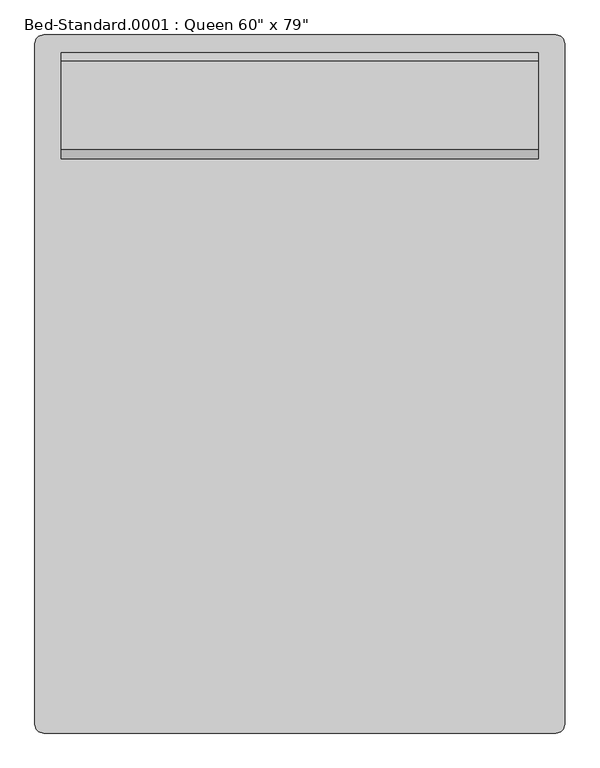
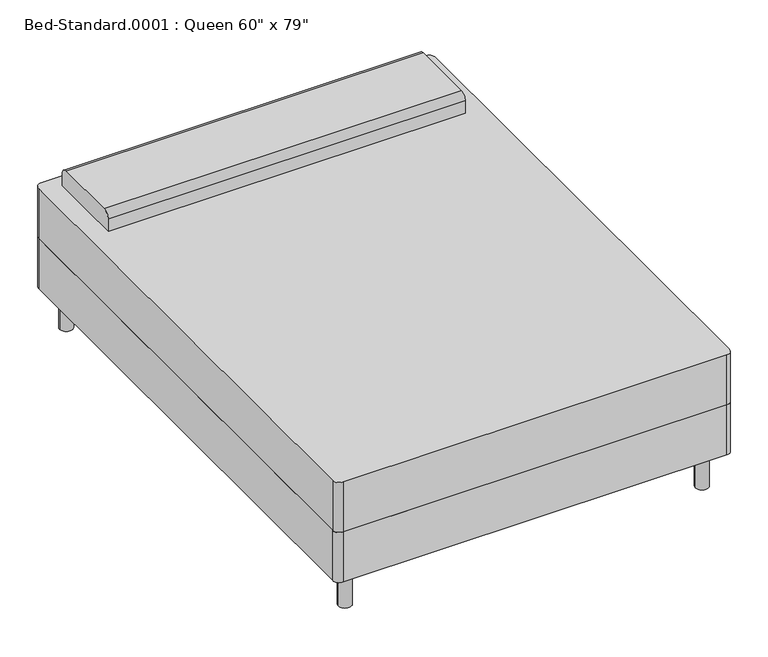
"""IFC4 building model written with IfcOpenShell, lengths in millimetres: furniture geometry."""

from ifc_helpers import new_model, si_unit, point, frame, frame_2d, origin, origin_with_axes, place, context, project, spatial, polyline, circle_curve, trimmed, segment, composite_curve, outline, extrude, source, transform, mapped, element, save


def furniture_e1791683(model_context):
    return source(origin(), model_context, "Body", "SweptSolid", [
        extrude(outline(composite_curve([segment(polyline([(-490.5114754, -1023.495082), (-490.5114754, 932.304918)]), True, "CONTINUOUS"), segment(trimmed(circle_curve(frame_2d((-465.1114754, 932.304918)), 25.4), [point((-490.5114754, 932.304918))], [point((-465.1114754, 957.704918))], False, "CARTESIAN"), True, "CONTINUOUS"), segment(polyline([(-465.1114754, 957.704918), (1008.0885246, 957.704918)]), True, "CONTINUOUS"), segment(trimmed(circle_curve(frame_2d((1008.0885246, 932.304918)), 25.4), [point((1008.0885246, 957.704918))], [point((1033.4885246, 932.304918))], False, "CARTESIAN"), True, "CONTINUOUS"), segment(polyline([(1033.4885246, 932.304918), (1033.4885246, -1023.495082)]), True, "CONTINUOUS"), segment(trimmed(circle_curve(frame_2d((1008.0885246, -1023.495082)), 25.4), [point((1033.4885246, -1023.495082))], [point((1008.0885246, -1048.895082))], False, "CARTESIAN"), True, "CONTINUOUS"), segment(polyline([(1008.0885246, -1048.895082), (-465.1114754, -1048.895082)]), True, "CONTINUOUS"), segment(trimmed(circle_curve(frame_2d((-465.1114754, -1023.495082)), 25.4), [point((-465.1114754, -1048.895082))], [point((-490.5114754, -1023.495082))], False, "CARTESIAN"), True, "CONTINUOUS")], self_intersect=False)), frame((0.0, 0.0, 152.4), z_axis=(0.0, 0.0, 1.0), x_axis=(1.0, 0.0, 0.0)), (0.0, 0.0, 1.0), 203.2),
        extrude(outline(composite_curve([segment(polyline([(602.104918, 558.8), (602.104918, 609.6)]), True, "CONTINUOUS"), segment(trimmed(circle_curve(frame_2d((627.504918, 609.6)), 25.4), [point((602.104918, 609.6))], [point((627.504918, 635.0))], False, "CARTESIAN"), True, "CONTINUOUS"), segment(polyline([(627.504918, 635.0), (881.504918, 635.0)]), True, "CONTINUOUS"), segment(trimmed(circle_curve(frame_2d((881.504918, 609.6)), 25.4), [point((881.504918, 635.0))], [point((906.904918, 609.6))], False, "CARTESIAN"), True, "CONTINUOUS"), segment(polyline([(906.904918, 609.6), (906.904918, 558.8), (602.104918, 558.8)]), True, "CONTINUOUS")], self_intersect=False)), frame((-414.3114754, 0.0, 0.0), z_axis=(1.0, 0.0, 0.0), x_axis=(0.0, 1.0, 0.0)), (0.0, 0.0, 1.0), 1371.6),
        extrude(outline(composite_curve([segment(trimmed(circle_curve(frame_2d((-414.3114754, 881.504918)), 25.4), [point((-439.7114754, 881.504918))], [point((-388.9114754, 881.504918))], False, "CARTESIAN"), True, "CONTINUOUS"), segment(trimmed(circle_curve(frame_2d((-414.3114754, 881.504918)), 25.4), [point((-388.9114754, 881.504918))], [point((-439.7114754, 881.504918))], False, "CARTESIAN"), True, "CONTINUOUS")], self_intersect=False)), origin_with_axes(), (0.0, 0.0, 1.0), 152.4),
        extrude(outline(composite_curve([segment(trimmed(circle_curve(frame_2d((957.2885246, 881.504918)), 25.4), [point((931.8885246, 881.504918))], [point((982.6885246, 881.504918))], False, "CARTESIAN"), True, "CONTINUOUS"), segment(trimmed(circle_curve(frame_2d((957.2885246, 881.504918)), 25.4), [point((982.6885246, 881.504918))], [point((931.8885246, 881.504918))], False, "CARTESIAN"), True, "CONTINUOUS")], self_intersect=False)), origin_with_axes(), (0.0, 0.0, 1.0), 152.4),
        extrude(outline(composite_curve([segment(trimmed(circle_curve(frame_2d((957.2885246, -972.695082)), 25.4), [point((931.8885246, -972.695082))], [point((982.6885246, -972.695082))], False, "CARTESIAN"), True, "CONTINUOUS"), segment(trimmed(circle_curve(frame_2d((957.2885246, -972.695082)), 25.4), [point((982.6885246, -972.695082))], [point((931.8885246, -972.695082))], False, "CARTESIAN"), True, "CONTINUOUS")], self_intersect=False)), origin_with_axes(), (0.0, 0.0, 1.0), 152.4),
        extrude(outline(composite_curve([segment(trimmed(circle_curve(frame_2d((-414.3114754, -972.695082)), 25.4), [point((-439.7114754, -972.695082))], [point((-388.9114754, -972.695082))], False, "CARTESIAN"), True, "CONTINUOUS"), segment(trimmed(circle_curve(frame_2d((-414.3114754, -972.695082)), 25.4), [point((-388.9114754, -972.695082))], [point((-439.7114754, -972.695082))], False, "CARTESIAN"), True, "CONTINUOUS")], self_intersect=False)), origin_with_axes(), (0.0, 0.0, 1.0), 152.4),
        extrude(outline(composite_curve([segment(polyline([(-465.1114754, 957.704918), (1008.0885246, 957.704918)]), True, "CONTINUOUS"), segment(trimmed(circle_curve(frame_2d((1008.0885246, 932.304918)), 25.4), [point((1008.0885246, 957.704918))], [point((1033.4885246, 932.304918))], False, "CARTESIAN"), True, "CONTINUOUS"), segment(polyline([(1033.4885246, 932.304918), (1033.4885246, -1023.495082)]), True, "CONTINUOUS"), segment(trimmed(circle_curve(frame_2d((1008.0885246, -1023.495082)), 25.4), [point((1033.4885246, -1023.495082))], [point((1008.0885246, -1048.895082))], False, "CARTESIAN"), True, "CONTINUOUS"), segment(polyline([(1008.0885246, -1048.895082), (-465.1114754, -1048.895082)]), True, "CONTINUOUS"), segment(trimmed(circle_curve(frame_2d((-465.1114754, -1023.495082)), 25.4), [point((-465.1114754, -1048.895082))], [point((-490.5114754, -1023.495082))], False, "CARTESIAN"), True, "CONTINUOUS"), segment(polyline([(-490.5114754, -1023.495082), (-490.5114754, 932.304918)]), True, "CONTINUOUS"), segment(trimmed(circle_curve(frame_2d((-465.1114754, 932.304918)), 25.4), [point((-490.5114754, 932.304918))], [point((-465.1114754, 957.704918))], False, "CARTESIAN"), True, "CONTINUOUS")], self_intersect=False)), frame((0.0, 0.0, 355.6), z_axis=(0.0, 0.0, 1.0), x_axis=(1.0, 0.0, 0.0)), (0.0, 0.0, 1.0), 203.2),
    ])


if __name__ == "__main__":
    model = new_model("IFC4")
    model_context = context("Model", 3, world=origin())
    ifc_project = project(units=[si_unit("LENGTHUNIT", "METRE", prefix="MILLI")], contexts=[model_context])
    site = spatial("IfcSite", under=ifc_project)
    building = spatial("IfcBuilding", under=site)
    placement = place(None, origin())
    furniture_shape = furniture_e1791683(model_context)
    element("IfcFurniture", 1, ObjectType="Bed-Standard.0001 : Queen 60\" x 79\"", at=placement, inside=building, context=model_context, shape_type="MappedRepresentation", body=[
        mapped(furniture_shape, transform((0.0, 0.0, 0.0), x_axis=(1.0, 0.0, 0.0), y_axis=(0.0, 1.0, 0.0), z_axis=(0.0, 0.0, 1.0))),
    ])
    save(model, "model.ifc")

# Revit data of these elements
# Type "Bed-Standard.0001 : Queen 60\" x 79\""
#   Assembly Code = "E2020200"
#   Length = 6' - 7"
#   Width = 5' - 0"
#   Leg Material = Steel, Chrome Plated
#   Mattress Material = Sash
#   Default Elevation = 0
# Element 1 (IfcFurniture, "Bed-Standard.0001 : Queen 60\" x 79\"")
#   Materials on its faces: "Linen, White", "Steel, Chrome Plated"
# Materials
#   "Steel, Chrome Plated": class "Metal", colour RGB 17 17 17, transparency 0, Description = "Chromiuim plated steel", Cost = 0
#   "Sash": class "Wood", colour RGB 224 178 126, transparency 0
#   "Linen, White": class "Textile", colour RGB 247 247 239, transparency 0, Description = "Linen, white", Cost = 0
